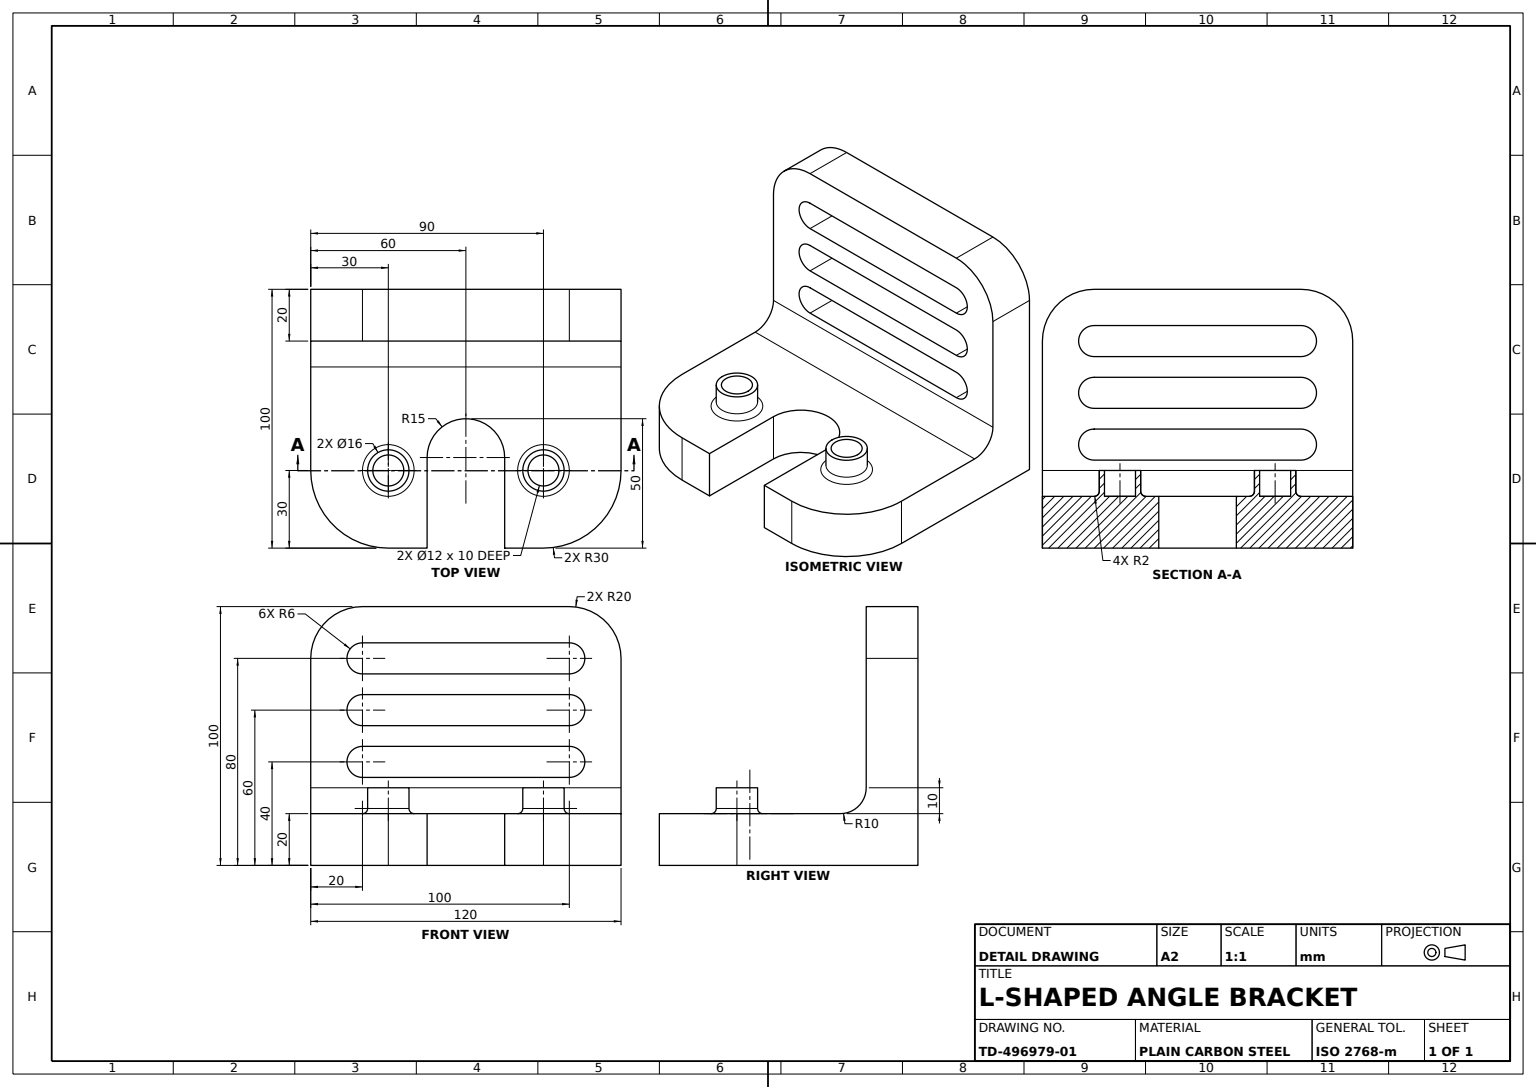
from build123d import *

# Parameters (mm, degrees)
BRACKET_BODY_DEPTH     = 60
CORNER_FILLET_R30_R    = 30
CORNER_FILLET_R20_R    = 20
BASE_NOTCH_DEPTH       = 78
UPRIGHT_SLOTS_3X_DEPTH = 20
BASE_BOSSES_PROFILE_R  = 8
BASE_BOSSES_2X_DEPTH   = 10
BOSS_EDGE_FILLET_R2_R  = 2
BOSS_HOLES_PROFILE_R   = 6
BOSS_HOLES_2X_DEPTH    = 10


with BuildPart() as part:
    # Bracket L Profile → Bracket Body (new, symmetric)
    with BuildSketch(Plane.XY):
        with BuildLine():
            Line((20, 0), (0, 0))
            Line((0, 0), (0, -80))
            Line((0, -80), (0, -100))
            Line((0, -100), (20, -100))
            Line((20, -100), (100, -100))
            Line((100, -100), (100, -80))
            Line((100, -80), (30, -80))
            ThreePointArc((30, -80), (22.928932188, -77.071067812), (20, -70))
            Line((20, -70), (20, 0))
        make_face()
    extrude(amount=BRACKET_BODY_DEPTH, both=True)

    # Corner Fillet R30
    corner_fillet_r30_edges = [part.edges().sort_by_distance(p)[0] for p in [
        (100, -90, 60),
        (100, -90, -60),
    ]]
    fillet(corner_fillet_r30_edges, radius=CORNER_FILLET_R30_R)

    # Corner Fillet R20
    corner_fillet_r20_edges = [part.edges().sort_by_distance(p)[0] for p in [
        (10, 0, -60),
        (10, 0, 60),
    ]]
    fillet(corner_fillet_r20_edges, radius=CORNER_FILLET_R20_R)

    # Base Notch Profile → Base Notch (cut)
    with BuildSketch(Plane(origin=(0, -80, 0), x_dir=(1, 0, 0), z_dir=(0, 1, 0))):
        with BuildLine():
            Line((65, 15), (100, 15))
            Line((100, 15), (100, -15))
            Line((100, -15), (65, -15))
            ThreePointArc((65, -15), (50, 0), (65, 15))
        make_face()
    extrude(amount=-BASE_NOTCH_DEPTH, mode=Mode.SUBTRACT)

    # Upright Slots Profile → Upright Slots 3x (cut)
    with BuildSketch(Plane(origin=(20, 0, 0), x_dir=(0, 0, -1), z_dir=(1, 0, 0))):
        with BuildLine():
            Line((-40, -14), (40, -14))
            ThreePointArc((40, -14), (46, -20), (40, -26))
            Line((40, -26), (-40, -26))
            ThreePointArc((-40, -26), (-46, -20), (-40, -14))
        make_face()
        with BuildLine():
            Line((-40, -46), (40, -46))
            ThreePointArc((40, -46), (46, -40), (40, -34))
            Line((40, -34), (-40, -34))
            ThreePointArc((-40, -34), (-46, -40), (-40, -46))
        make_face()
        with BuildLine():
            Line((-40, -66), (40, -66))
            ThreePointArc((40, -66), (46, -60), (40, -54))
            Line((40, -54), (-40, -54))
            ThreePointArc((-40, -54), (-46, -60), (-40, -66))
        make_face()
    extrude(amount=-UPRIGHT_SLOTS_3X_DEPTH, mode=Mode.SUBTRACT)

    # Base Bosses Profile → Base Bosses 2x (add)
    with BuildSketch(Plane(origin=(0, -80, 0), x_dir=(1, 0, 0), z_dir=(0, 1, 0))):
        with Locations(Location((70, 30, 0), (0, 0, 270))):
            Circle(BASE_BOSSES_PROFILE_R)
        with Locations(Location((70, -30, 0), (0, 0, 270))):
            Circle(BASE_BOSSES_PROFILE_R)
    extrude(amount=BASE_BOSSES_2X_DEPTH)

    # Boss Edge Fillet R2
    boss_edge_fillet_r2_edges = [part.edges().sort_by_distance(p)[0] for p in [
        (70, -80, -38),
        (70, -80, 22),
    ]]
    fillet(boss_edge_fillet_r2_edges, radius=BOSS_EDGE_FILLET_R2_R)

    # Boss Holes Profile → Boss Holes 2x (cut)
    with BuildSketch(Plane(origin=(0, -70, 0), x_dir=(1, 0, 0), z_dir=(0, 1, 0))):
        with Locations(Location((70, -30, 0), (0, 0, 270))):
            Circle(BOSS_HOLES_PROFILE_R)
        with Locations(Location((70, 30, 0), (0, 0, 270))):
            Circle(BOSS_HOLES_PROFILE_R)
    extrude(amount=-BOSS_HOLES_2X_DEPTH, mode=Mode.SUBTRACT)


solid = part.part
